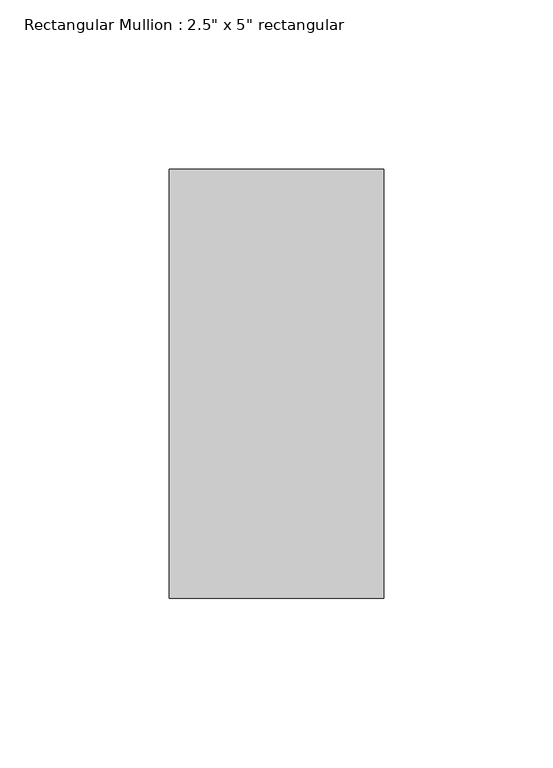
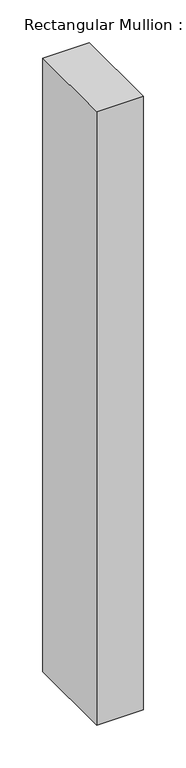
"""IFC4 building model written with IfcOpenShell, lengths in millimetres: member geometry."""

from ifc_helpers import new_model, si_unit, frame, origin, place, context, project, spatial, polyline, outline, extrude, source, transform, mapped, element, save


def member_b96be9f2(model_context):
    return source(origin(), model_context, "Body", "SweptSolid", [
        extrude(outline(polyline([(31.75, 63.5), (31.75, -63.5), (-31.75, -63.5), (-31.75, 63.5), (31.75, 63.5)])), frame((0.0, 0.0, -880.2652244), z_axis=(0.0, 0.0, 1.0), x_axis=(1.0, 0.0, 0.0)), (0.0, 0.0, 1.0), 880.2652244),
    ])


if __name__ == "__main__":
    model = new_model("IFC4")
    model_context = context("Model", 3, world=origin())
    ifc_project = project(units=[si_unit("LENGTHUNIT", "METRE", prefix="MILLI")], contexts=[model_context])
    site = spatial("IfcSite", under=ifc_project)
    building = spatial("IfcBuilding", under=site)
    placement = place(None, origin())
    member_shape = member_b96be9f2(model_context)
    element("IfcMember", 1, ObjectType="Rectangular Mullion : 2.5\" x 5\" rectangular", at=placement, inside=building, context=model_context, shape_type="MappedRepresentation", body=[
        mapped(member_shape, transform((0.0, 0.0, 0.0), x_axis=(1.0, 0.0, 0.0), y_axis=(0.0, 1.0, 0.0), z_axis=(0.0, 0.0, 1.0))),
    ])
    save(model, "model.ifc")

# Revit data of these elements
# Type "Rectangular Mullion : 2.5\" x 5\" rectangular"
#   built-in parameter 1007304 = 0.416667 (stored number, unit not read)
#   built-in parameter 1007301 = 0.104167 (stored number, unit not read)
#   built-in parameter 1007300 = 0.104167 (stored number, unit not read)
# Element 1 (IfcMember, "Rectangular Mullion : 2.5\" x 5\" rectangular")
#   Materials on its faces: "Aluminum"
# Materials
#   "Aluminum": class "Metal", colour RGB 247 247 247, transparency 0, Description = "Aluminum 6061", Cost = 0
